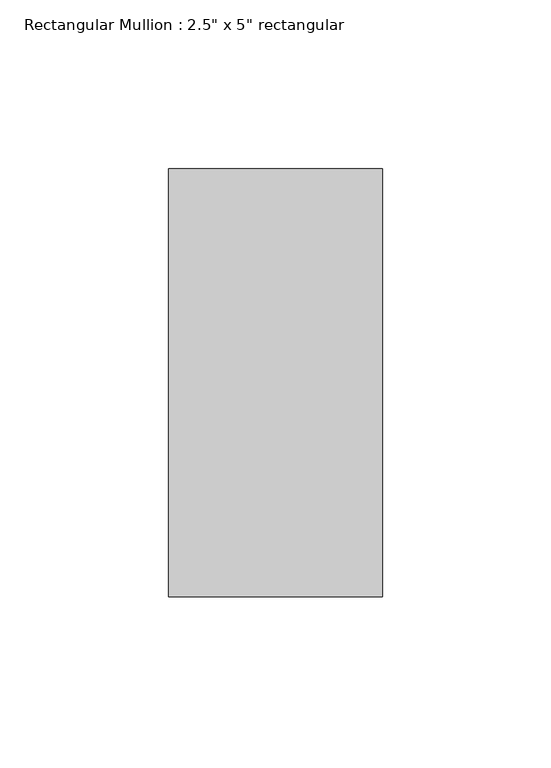
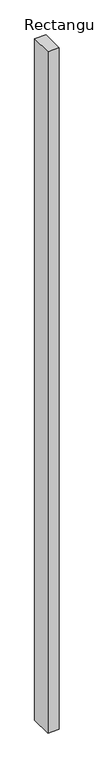
"""IFC4 building model written with IfcOpenShell, lengths in millimetres: member geometry."""

from ifc_helpers import new_model, si_unit, frame, origin, place, context, project, spatial, polyline, outline, extrude, source, transform, mapped, element, save


def member_20b53a5f(model_context):
    return source(origin(), model_context, "Body", "SweptSolid", [
        extrude(outline(polyline([(0.0, 63.5), (0.0, -63.5), (-63.5, -63.5), (-63.5, 63.5), (0.0, 63.5)])), frame((0.0, 0.0, -4019.55), z_axis=(0.0, 0.0, 1.0), x_axis=(1.0, 0.0, 0.0)), (0.0, 0.0, 1.0), 4019.55),
    ])


if __name__ == "__main__":
    model = new_model("IFC4")
    model_context = context("Model", 3, world=origin())
    ifc_project = project(units=[si_unit("LENGTHUNIT", "METRE", prefix="MILLI")], contexts=[model_context])
    site = spatial("IfcSite", under=ifc_project)
    building = spatial("IfcBuilding", under=site)
    placement = place(None, origin())
    member_shape = member_20b53a5f(model_context)
    element("IfcMember", 1, ObjectType="Rectangular Mullion : 2.5\" x 5\" rectangular", at=placement, inside=building, context=model_context, shape_type="MappedRepresentation", body=[
        mapped(member_shape, transform((0.0, 0.0, 0.0), x_axis=(1.0, 0.0, 0.0), y_axis=(0.0, 1.0, 0.0), z_axis=(0.0, 0.0, 1.0))),
    ])
    save(model, "model.ifc")

# Revit data of these elements
# Type "Rectangular Mullion : 2.5\" x 5\" rectangular"
#   built-in parameter 1007304 = 0.416667 (stored number, unit not read)
#   built-in parameter 1007301 = 0.104167 (stored number, unit not read)
#   built-in parameter 1007300 = 0.104167 (stored number, unit not read)
# Element 1 (IfcMember, "Rectangular Mullion : 2.5\" x 5\" rectangular")
#   Materials on its faces: "Iron, Ductile"
# Materials
#   "Iron, Ductile": class "Metal", colour RGB 0 0 0, transparency 0, Description = "Ductile cast iron", Cost = 0
